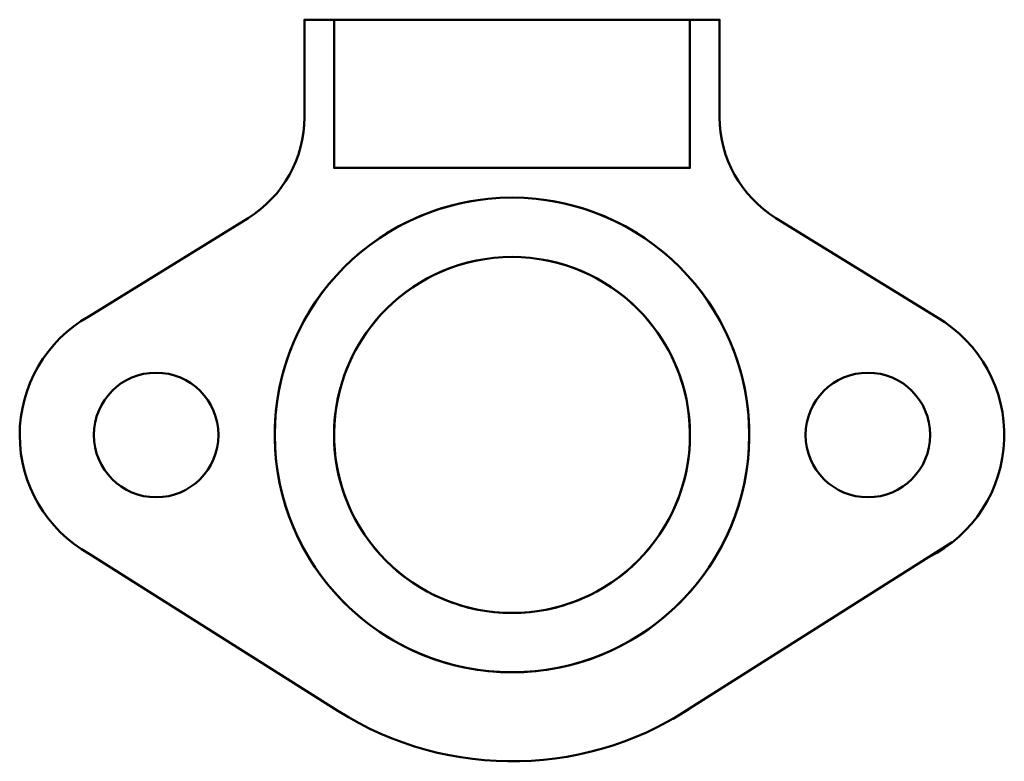
# Model space of a CAD drawing. Units: millimetres. Extents: x 2994 to 3160, y 1466 to 1591.
import ezdxf

# ---------------------------------------------------------------- set-up
doc = ezdxf.new("R2010")
doc.units = ezdxf.units.MM
doc.layers.add('M-OUTL', color=7, linetype='Continuous', lineweight=50)

msp = doc.modelspace()

# ---------------------------------------------------------------- linework, layer by layer
at = {"layer": 'M-OUTL'}
for p, q in [((3082.04, 1565.8), (3107.04, 1565.8)), ((3151.25, 1502.72), (3104.2, 1472.98))]:
    msp.add_line(p, q, dxfattribs=at)
msp.add_lwpolyline([(3147.27, 1500.2, 0.595906), (3148.68, 1540.63), (3121.54, 1557.36, -0.260226), (3112.04, 1574.39), (3112.04, 1590.8), (3042.04, 1590.8), (3042.04, 1574.39, -0.26017), (3032.54, 1557.36), (3005.67, 1540.79, 0.583328), (3005.76, 1500.75), (3047.68, 1474.29, 0.302202), (3108.58, 1475.74)], format="xyb", dxfattribs=at)
for points in [[(3047.04, 1565.8), (3107.04, 1565.8), (3107.04, 1590.8), (3112.04, 1590.8)], [(3072.04, 1565.8), (3047.04, 1565.8), (3047.04, 1590.8), (3107.04, 1590.8)]]:
    msp.add_lwpolyline(points, dxfattribs=at)
at = {"layer": 'M-OUTL', "extrusion": (0, 1, 0)}
msp.add_circle((-3077.04, 15, 1565.8), 5, dxfattribs=at)
at = {"layer": 'M-OUTL'}
for centre, radius in [((3077.04, 1520.8), 40), ((3077.04, 1520.8), 30), ((3017.04, 1520.8), 10.5), ((3137.04, 1520.8), 10.5)]:
    msp.add_circle(centre, radius, dxfattribs=at)
for radius, start, end in [(40, 97.1808, 82.8192), (30, 99.5941, 80.4059)]:
    msp.add_arc((3077.04, 1520.8), radius, start, end, dxfattribs=at)

doc.saveas('drawing.dxf')
